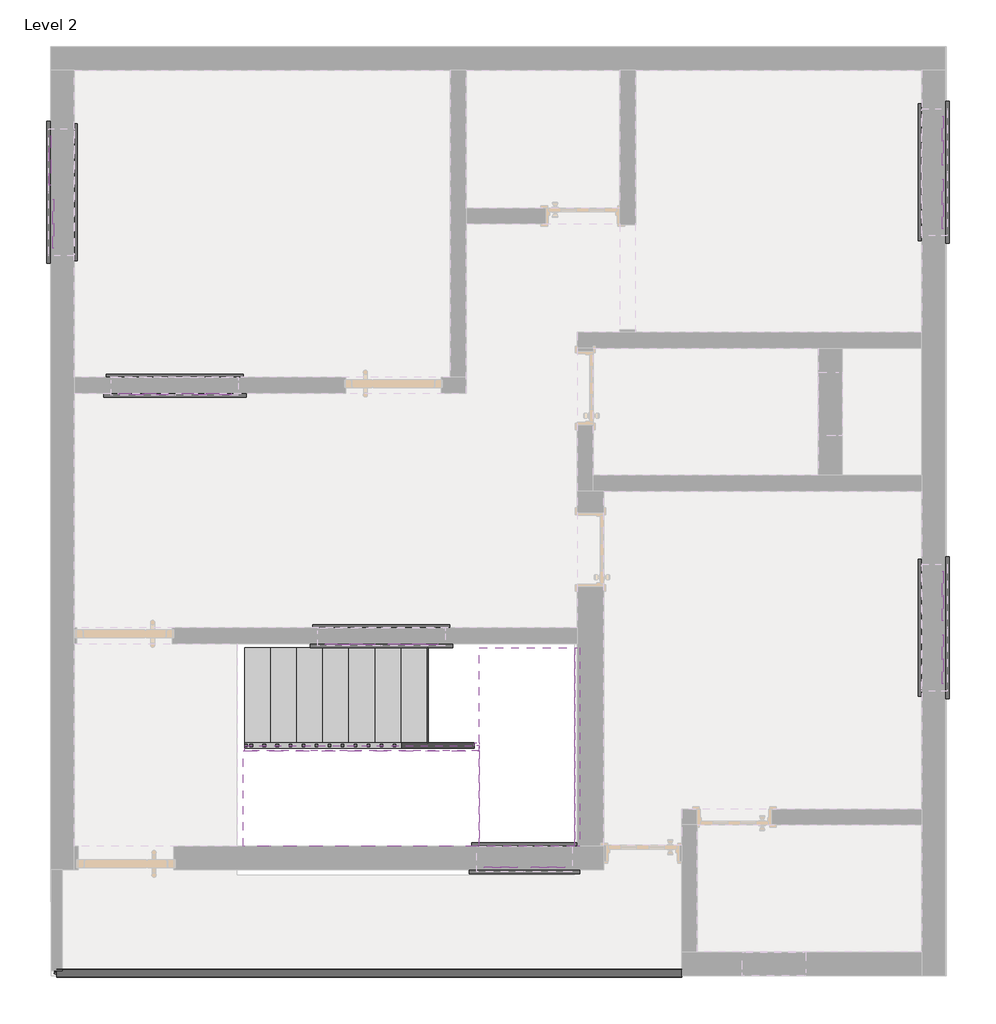
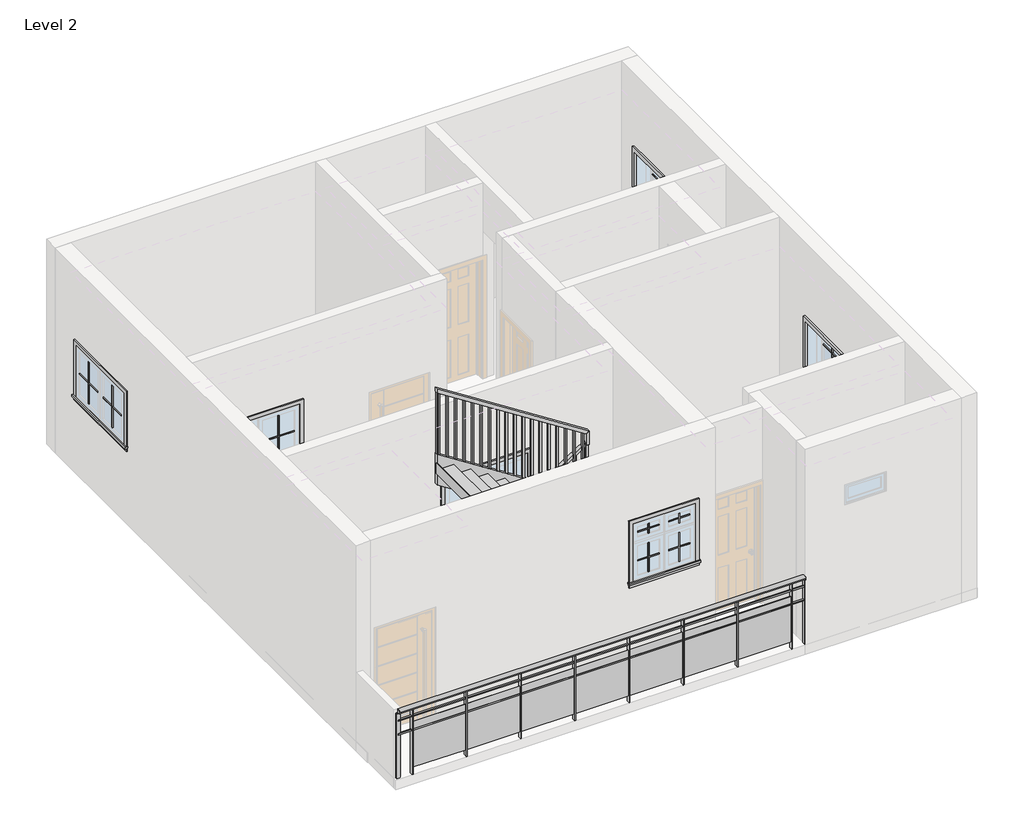
# One storey, part 2 of 2: 26 proxies, 4 members, 2 railings, 2 stair flights, 1 slab.
"""IFC4 building model written with IfcOpenShell, lengths in millimetres."""

from ifc_helpers import new_model, si_unit, point, frame, origin, place, context, project, spatial, polyline, ellipse_curve, trimmed, outline, extrude, faceted_brep, transform, mapped, element, save
from ifc_brep_helpers import plane_surface, extruded_surface, advanced_brep
from components import m_muntin_pattern_2x2_m_muntin_pattern_2x2_8d9e5da3, m_muntin_pattern_2x2_m_muntin_pattern_2x2_32a0f80e, m_muntin_pattern_2x2_m_muntin_pattern_2x2_5c9fa27a, m_muntin_pattern_2x2_m_muntin_pattern_2x2_8c7fd3cb, m_muntin_pattern_2x2_m_muntin_pattern_2x2_332c70e0, m_trim_window_exterior_flat_with_sill_3a557199, m_trim_window_exterior_flat_with_sill_8fa486dc, m_trim_window_interior_flat_picture_frame_580345df, m_trim_window_interior_flat_picture_frame_b6dd03a6, non_monolithic_landing_e1259e21, stair_flight_50mm_tread_13mm_riser_06224c7e, stair_flight_50mm_tread_13mm_riser_05b05da2

model = new_model("IFC4")

# Units and contexts
model_context = context("Model", 3, world=origin())
ifc_project = project(units=[si_unit("LENGTHUNIT", "METRE", prefix="MILLI")], contexts=[model_context])

# Site, building, storey
site = spatial("IfcSite", under=ifc_project)
building = spatial("IfcBuilding", under=site)
storey = spatial("IfcBuildingStorey", under=building, Name="Level 2", Elevation=3200.4)

# Proxies
placement = place(None, origin())
m_muntin_pattern_2x2_m_muntin_pattern_2x2_shape = m_muntin_pattern_2x2_m_muntin_pattern_2x2_8d9e5da3(model_context)
element("IfcBuildingElementProxy", 1, Name="M_Muntin Pattern_2x2 : M_Muntin Pattern_2x2", ObjectType="M_Muntin Pattern_2x2 : M_Muntin Pattern_2x2", at=placement, inside=storey, context=model_context, shape_type="MappedRepresentation", body=[
    mapped(m_muntin_pattern_2x2_m_muntin_pattern_2x2_shape, transform((-3082.7532945, -1629.5296603, 4489.45), x_axis=(0.0, -1.0, 0.0), y_axis=(1.0, 0.0, 0.0), z_axis=(0.0, 0.0, 1.0))),
])
element("IfcBuildingElementProxy", 2, Name="M_Muntin Pattern_2x2 : M_Muntin Pattern_2x2", ObjectType="M_Muntin Pattern_2x2 : M_Muntin Pattern_2x2", at=placement, inside=storey, context=model_context, shape_type="MappedRepresentation", body=[
    mapped(m_muntin_pattern_2x2_m_muntin_pattern_2x2_shape, transform((-3082.7532945, 2739.2703397, 4489.45), x_axis=(0.0, -1.0, 0.0), y_axis=(1.0, 0.0, 0.0), z_axis=(0.0, 0.0, 1.0))),
])
element("IfcBuildingElementProxy", 3, Name="M_Muntin Pattern_2x2 : M_Muntin Pattern_2x2", ObjectType="M_Muntin Pattern_2x2 : M_Muntin Pattern_2x2", at=placement, inside=storey, context=model_context, shape_type="MappedRepresentation", body=[
    mapped(m_muntin_pattern_2x2_m_muntin_pattern_2x2_shape, transform((-10161.4157945, 324.6828397, 4489.45), x_axis=(-1.0, 0.0, 0.0), y_axis=(0.0, -1.0, 0.0), z_axis=(0.0, 0.0, 1.0))),
])
element("IfcBuildingElementProxy", 4, Name="M_Muntin Pattern_2x2 : M_Muntin Pattern_2x2", ObjectType="M_Muntin Pattern_2x2 : M_Muntin Pattern_2x2", at=placement, inside=storey, context=model_context, shape_type="MappedRepresentation", body=[
    mapped(m_muntin_pattern_2x2_m_muntin_pattern_2x2_shape, transform((-11648.9032945, 1942.3453397, 4489.45), x_axis=(0.0, 1.0, 0.0), y_axis=(-1.0, 0.0, 0.0), z_axis=(0.0, 0.0, 1.0))),
])
element("IfcBuildingElementProxy", 5, Name="M_Muntin Pattern_2x2 : M_Muntin Pattern_2x2", ObjectType="M_Muntin Pattern_2x2 : M_Muntin Pattern_2x2", at=placement, inside=storey, context=model_context, shape_type="MappedRepresentation", body=[
    mapped(m_muntin_pattern_2x2_m_muntin_pattern_2x2_shape, transform((-8180.2157945, -2075.6171603, 4489.45), x_axis=(-1.0, 0.0, 0.0), y_axis=(0.0, -1.0, 0.0), z_axis=(0.0, 0.0, 1.0))),
])
m_muntin_pattern_2x2_m_muntin_pattern_2x2_2_shape = m_muntin_pattern_2x2_m_muntin_pattern_2x2_32a0f80e(model_context)
element("IfcBuildingElementProxy", 6, Name="M_Muntin Pattern_2x2 : M_Muntin Pattern_2x2", ObjectType="M_Muntin Pattern_2x2 : M_Muntin Pattern_2x2", at=placement, inside=storey, context=model_context, shape_type="MappedRepresentation", body=[
    mapped(m_muntin_pattern_2x2_m_muntin_pattern_2x2_2_shape, transform((-3082.7532945, -2235.9546603, 4489.45), x_axis=(0.0, 1.0, 0.0), y_axis=(-1.0, 0.0, 0.0), z_axis=(0.0, 0.0, 1.0))),
])
element("IfcBuildingElementProxy", 7, Name="M_Muntin Pattern_2x2 : M_Muntin Pattern_2x2", ObjectType="M_Muntin Pattern_2x2 : M_Muntin Pattern_2x2", at=placement, inside=storey, context=model_context, shape_type="MappedRepresentation", body=[
    mapped(m_muntin_pattern_2x2_m_muntin_pattern_2x2_2_shape, transform((-3082.7532945, 2132.8453397, 4489.45), x_axis=(0.0, 1.0, 0.0), y_axis=(-1.0, 0.0, 0.0), z_axis=(0.0, 0.0, 1.0))),
])
element("IfcBuildingElementProxy", 8, Name="M_Muntin Pattern_2x2 : M_Muntin Pattern_2x2", ObjectType="M_Muntin Pattern_2x2 : M_Muntin Pattern_2x2", at=placement, inside=storey, context=model_context, shape_type="MappedRepresentation", body=[
    mapped(m_muntin_pattern_2x2_m_muntin_pattern_2x2_2_shape, transform((-10767.8407945, 324.6828397, 4489.45), x_axis=(1.0, 0.0, 0.0), y_axis=(0.0, 1.0, 0.0), z_axis=(0.0, 0.0, 1.0))),
])
element("IfcBuildingElementProxy", 9, Name="M_Muntin Pattern_2x2 : M_Muntin Pattern_2x2", ObjectType="M_Muntin Pattern_2x2 : M_Muntin Pattern_2x2", at=placement, inside=storey, context=model_context, shape_type="MappedRepresentation", body=[
    mapped(m_muntin_pattern_2x2_m_muntin_pattern_2x2_2_shape, transform((-11648.9032945, 2548.7703397, 4489.45), x_axis=(0.0, -1.0, 0.0), y_axis=(1.0, 0.0, 0.0), z_axis=(0.0, 0.0, 1.0))),
])
element("IfcBuildingElementProxy", 10, Name="M_Muntin Pattern_2x2 : M_Muntin Pattern_2x2", ObjectType="M_Muntin Pattern_2x2 : M_Muntin Pattern_2x2", at=placement, inside=storey, context=model_context, shape_type="MappedRepresentation", body=[
    mapped(m_muntin_pattern_2x2_m_muntin_pattern_2x2_2_shape, transform((-8786.6407945, -2075.6171603, 4489.45), x_axis=(1.0, 0.0, 0.0), y_axis=(0.0, 1.0, 0.0), z_axis=(0.0, 0.0, 1.0))),
])
m_muntin_pattern_2x2_m_muntin_pattern_2x2_3_shape = m_muntin_pattern_2x2_m_muntin_pattern_2x2_5c9fa27a(model_context)
element("IfcBuildingElementProxy", 11, Name="M_Muntin Pattern_2x2 : M_Muntin Pattern_2x2", ObjectType="M_Muntin Pattern_2x2 : M_Muntin Pattern_2x2", at=placement, inside=storey, context=model_context, shape_type="MappedRepresentation", body=[
    mapped(m_muntin_pattern_2x2_m_muntin_pattern_2x2_3_shape, transform((-6884.8157945, -4247.3171603, 4489.45), x_axis=(-1.0, 0.0, 0.0), y_axis=(0.0, -1.0, 0.0), z_axis=(0.0, 0.0, 1.0))),
])
m_muntin_pattern_2x2_m_muntin_pattern_2x2_4_shape = m_muntin_pattern_2x2_m_muntin_pattern_2x2_8c7fd3cb(model_context)
element("IfcBuildingElementProxy", 12, Name="M_Muntin Pattern_2x2 : M_Muntin Pattern_2x2", ObjectType="M_Muntin Pattern_2x2 : M_Muntin Pattern_2x2", at=placement, inside=storey, context=model_context, shape_type="MappedRepresentation", body=[
    mapped(m_muntin_pattern_2x2_m_muntin_pattern_2x2_4_shape, transform((-7338.8407945, -4247.3171603, 4489.45), x_axis=(1.0, 0.0, 0.0), y_axis=(0.0, 1.0, 0.0), z_axis=(0.0, 0.0, 1.0))),
])
m_muntin_pattern_2x2_m_muntin_pattern_2x2_5_shape = m_muntin_pattern_2x2_m_muntin_pattern_2x2_332c70e0(model_context)
element("IfcBuildingElementProxy", 13, Name="M_Muntin Pattern_2x2 : M_Muntin Pattern_2x2", ObjectType="M_Muntin Pattern_2x2 : M_Muntin Pattern_2x2", at=placement, inside=storey, context=model_context, shape_type="MappedRepresentation", body=[
    mapped(m_muntin_pattern_2x2_m_muntin_pattern_2x2_5_shape, transform((-7338.8407945, -4247.3171603, 5089.45), x_axis=(1.0, 0.0, 0.0), y_axis=(0.0, 1.0, 0.0), z_axis=(0.0, 0.0, 1.0))),
])
element("IfcBuildingElementProxy", 14, Name="M_Muntin Pattern_2x2 : M_Muntin Pattern_2x2", ObjectType="M_Muntin Pattern_2x2 : M_Muntin Pattern_2x2", at=placement, inside=storey, context=model_context, shape_type="MappedRepresentation", body=[
    mapped(m_muntin_pattern_2x2_m_muntin_pattern_2x2_5_shape, transform((-6884.8157945, -4247.3171603, 5089.45), x_axis=(1.0, 0.0, 0.0), y_axis=(0.0, 1.0, 0.0), z_axis=(0.0, 0.0, 1.0))),
])
m_trim_window_exterior_flat_with_sill_shape = m_trim_window_exterior_flat_with_sill_3a557199(model_context)
element("IfcBuildingElementProxy", 15, Name="M_Trim-Window-Exterior-Flat : with Sill", ObjectType="M_Trim-Window-Exterior-Flat : with Sill", at=placement, inside=storey, context=model_context, shape_type="MappedRepresentation", body=[
    mapped(m_trim_window_exterior_flat_with_sill_shape, transform((-3073.2282945, -1932.7421603, 5219.6), x_axis=(0.0, 1.0, 0.0), y_axis=(0.0, 0.0, 1.0), z_axis=(1.0, 0.0, 0.0))),
])
element("IfcBuildingElementProxy", 16, Name="M_Trim-Window-Exterior-Flat : with Sill", ObjectType="M_Trim-Window-Exterior-Flat : with Sill", at=placement, inside=storey, context=model_context, shape_type="MappedRepresentation", body=[
    mapped(m_trim_window_exterior_flat_with_sill_shape, transform((-3073.2282945, 2436.0578397, 5219.6), x_axis=(0.0, 1.0, 0.0), y_axis=(0.0, 0.0, 1.0), z_axis=(1.0, 0.0, 0.0))),
])
element("IfcBuildingElementProxy", 17, Name="M_Trim-Window-Exterior-Flat : with Sill", ObjectType="M_Trim-Window-Exterior-Flat : with Sill", at=placement, inside=storey, context=model_context, shape_type="MappedRepresentation", body=[
    mapped(m_trim_window_exterior_flat_with_sill_shape, transform((-10464.6282945, 315.1578397, 5219.6), x_axis=(1.0, 0.0, 0.0), y_axis=(0.0, 0.0, 1.0), z_axis=(0.0, -1.0, 0.0))),
])
element("IfcBuildingElementProxy", 18, Name="M_Trim-Window-Exterior-Flat : with Sill", ObjectType="M_Trim-Window-Exterior-Flat : with Sill", at=placement, inside=storey, context=model_context, shape_type="MappedRepresentation", body=[
    mapped(m_trim_window_exterior_flat_with_sill_shape, transform((-11658.4282945, 2245.5578397, 5219.6), x_axis=(0.0, -1.0, 0.0), y_axis=(0.0, 0.0, 1.0), z_axis=(-1.0, 0.0, 0.0))),
])
element("IfcBuildingElementProxy", 19, Name="M_Trim-Window-Exterior-Flat : with Sill", ObjectType="M_Trim-Window-Exterior-Flat : with Sill", at=placement, inside=storey, context=model_context, shape_type="MappedRepresentation", body=[
    mapped(m_trim_window_exterior_flat_with_sill_shape, transform((-8483.4282945, -2085.1421603, 5219.6), x_axis=(1.0, 0.0, 0.0), y_axis=(0.0, 0.0, 1.0), z_axis=(0.0, -1.0, 0.0))),
])
m_trim_window_exterior_flat_with_sill_2_shape = m_trim_window_exterior_flat_with_sill_8fa486dc(model_context)
element("IfcBuildingElementProxy", 20, Name="M_Trim-Window-Exterior-Flat : with Sill", ObjectType="M_Trim-Window-Exterior-Flat : with Sill", at=placement, inside=storey, context=model_context, shape_type="MappedRepresentation", body=[
    mapped(m_trim_window_exterior_flat_with_sill_2_shape, transform((-7111.8282945, -4256.8421603, 5319.6), x_axis=(1.0, 0.0, 0.0), y_axis=(0.0, 0.0, 1.0), z_axis=(0.0, -1.0, 0.0))),
])
m_trim_window_interior_flat_picture_frame_shape = m_trim_window_interior_flat_picture_frame_580345df(model_context)
element("IfcBuildingElementProxy", 21, Name="M_Trim-Window-Interior-Flat : Picture Frame", ObjectType="M_Trim-Window-Interior-Flat : Picture Frame", at=placement, inside=storey, context=model_context, shape_type="MappedRepresentation", body=[
    mapped(m_trim_window_interior_flat_picture_frame_shape, transform((-3301.8282945, -1932.7421603, 5219.6), x_axis=(0.0, -1.0, 0.0), y_axis=(0.0, 0.0, 1.0), z_axis=(-1.0, 0.0, 0.0))),
])
element("IfcBuildingElementProxy", 22, Name="M_Trim-Window-Interior-Flat : Picture Frame", ObjectType="M_Trim-Window-Interior-Flat : Picture Frame", at=placement, inside=storey, context=model_context, shape_type="MappedRepresentation", body=[
    mapped(m_trim_window_interior_flat_picture_frame_shape, transform((-3301.8282945, 2436.0578397, 5219.6), x_axis=(0.0, -1.0, 0.0), y_axis=(0.0, 0.0, 1.0), z_axis=(-1.0, 0.0, 0.0))),
])
element("IfcBuildingElementProxy", 23, Name="M_Trim-Window-Interior-Flat : Picture Frame", ObjectType="M_Trim-Window-Interior-Flat : Picture Frame", at=placement, inside=storey, context=model_context, shape_type="MappedRepresentation", body=[
    mapped(m_trim_window_interior_flat_picture_frame_shape, transform((-10464.6282945, 467.5578397, 5219.6), x_axis=(-1.0, 0.0, 0.0), y_axis=(0.0, 0.0, 1.0), z_axis=(0.0, 1.0, 0.0))),
])
element("IfcBuildingElementProxy", 24, Name="M_Trim-Window-Interior-Flat : Picture Frame", ObjectType="M_Trim-Window-Interior-Flat : Picture Frame", at=placement, inside=storey, context=model_context, shape_type="MappedRepresentation", body=[
    mapped(m_trim_window_interior_flat_picture_frame_shape, transform((-11429.8282945, 2245.5578397, 5219.6), x_axis=(0.0, 1.0, 0.0), y_axis=(0.0, 0.0, 1.0), z_axis=(1.0, 0.0, 0.0))),
])
element("IfcBuildingElementProxy", 25, Name="M_Trim-Window-Interior-Flat : Picture Frame", ObjectType="M_Trim-Window-Interior-Flat : Picture Frame", at=placement, inside=storey, context=model_context, shape_type="MappedRepresentation", body=[
    mapped(m_trim_window_interior_flat_picture_frame_shape, transform((-8483.4282945, -1932.7421603, 5219.6), x_axis=(-1.0, 0.0, 0.0), y_axis=(0.0, 0.0, 1.0), z_axis=(0.0, 1.0, 0.0))),
])
m_trim_window_interior_flat_picture_frame_2_shape = m_trim_window_interior_flat_picture_frame_b6dd03a6(model_context)
element("IfcBuildingElementProxy", 26, Name="M_Trim-Window-Interior-Flat : Picture Frame", ObjectType="M_Trim-Window-Interior-Flat : Picture Frame", at=placement, inside=storey, context=model_context, shape_type="MappedRepresentation", body=[
    mapped(m_trim_window_interior_flat_picture_frame_2_shape, transform((-7111.8282945, -4028.2421603, 5319.6), x_axis=(-1.0, 0.0, 0.0), y_axis=(0.0, 0.0, 1.0), z_axis=(0.0, 1.0, 0.0))),
])

# Members
element("IfcMember", 27, ObjectType="Stringer - 50mm Width", at=placement, inside=storey, context=model_context, shape_type="SweptSolid", body=[
    extrude(outline(polyline([(3439.2262231, -9795.4329612), (3200.4, -9795.4329612), (3200.4, -9426.576984), (4372.4786661, -7595.4329612), (4847.4022231, -7595.4329612), (3439.2262231, -9795.4329612)])), frame((0.0, -3087.6421603, 0.0), z_axis=(0.0, 1.0, 0.0), x_axis=(0.0, 0.0, 1.0)), (0.0, 0.0, 1.0), 50.0),
])
element("IfcMember", 28, ObjectType="Stringer - 50mm Width", at=placement, inside=storey, context=model_context, shape_type="SweptSolid", body=[
    extrude(outline(polyline([(4564.5026661, -7545.4329612), (5039.4262231, -7545.4329612), (6479.6062231, -9795.4329612), (6004.6826661, -9795.4329612), (4564.5026661, -7545.4329612)])), frame((0.0, -3113.8421603, 0.0), z_axis=(0.0, 1.0, 0.0), x_axis=(0.0, 0.0, 1.0)), (0.0, 0.0, 1.0), 50.0),
])
element("IfcMember", 29, ObjectType="Stringer - 50mm Width", at=placement, inside=storey, context=model_context, shape_type="SweptSolid", body=[
    extrude(outline(polyline([(-6581.0329612, -4028.2421603), (-6631.0329612, -4028.2421603), (-6631.0329612, -2123.2421603), (-6581.0329612, -2123.2421603), (-6581.0329612, -4028.2421603)])), frame((0.0, 0.0, 4450.6), z_axis=(0.0, 0.0, 1.0), x_axis=(1.0, 0.0, 0.0)), (0.0, 0.0, 1.0), 400.0),
])
element("IfcMember", 30, ObjectType="Stringer - 50mm Width", at=placement, inside=storey, context=model_context, shape_type="SweptSolid", body=[
    extrude(outline(polyline([(-7595.4329612, -3037.6421603), (-7545.4329612, -3037.6421603), (-7545.4329612, -3063.8421603), (-7595.4329612, -3063.8421603), (-7595.4329612, -3037.6421603)])), frame((0.0, 0.0, 4450.6), z_axis=(0.0, 0.0, 1.0), x_axis=(1.0, 0.0, 0.0)), (0.0, 0.0, 1.0), 400.0),
])

# Railings
element("IfcRailing", 31, ObjectType="1100mm", at=placement, inside=storey, context=model_context, shape_type="SolidModel", body=[
    faceted_brep([(-9795.4329612, -3037.6421603, 4460.42), (-9795.4329612, -3037.6421603, 4401.0545554), (-9795.4329612, -3087.6421603, 4401.0545554), (-9795.4329612, -3087.6421603, 4460.42), (-7595.4329612, -3037.6421603, 5868.596), (-7595.4329612, -3087.6421603, 5868.596), (-7595.4329612, -3087.6421603, 5809.2305554), (-7595.4329612, -3037.6421603, 5809.2305554)], [[[0, 1, 2, 3]], [[4, 5, 6, 7]], [[1, 0, 4, 7]], [[2, 1, 7, 6]], [[3, 2, 6, 5]], [[0, 3, 5, 4]]]),
    faceted_brep([(-7545.4329612, -3037.6421603, 5900.6), (-7545.4329612, -3037.6421603, 5850.6), (-7595.4329612, -3037.6421603, 5850.6), (-7595.4329612, -3037.6421603, 5900.6), (-7545.4329612, -3063.8421603, 5900.6), (-7595.4329612, -3063.8421603, 5900.6), (-7595.4329612, -3113.8421603, 5850.6), (-7545.4329612, -3113.8421603, 5850.6)], [[[0, 1, 2, 3]], [[4, 5, 6, 7]], [[1, 0, 4, 7]], [[2, 1, 7, 6]], [[3, 2, 6, 5]], [[0, 3, 5, 4]]]),
    faceted_brep([(-7545.4329612, -3063.8421603, 5900.6), (-7545.4329612, -3113.8421603, 5850.6), (-7595.4329612, -3113.8421603, 5850.6), (-7595.4329612, -3063.8421603, 5900.6), (-7545.4329612, -3063.8421603, 6060.62), (-7595.4329612, -3063.8421603, 6033.2585554), (-7595.4329612, -3113.8421603, 6033.2585554), (-7545.4329612, -3113.8421603, 6060.62)], [[[0, 1, 2, 3]], [[4, 5, 6, 7]], [[1, 0, 4, 7]], [[2, 1, 7, 6]], [[3, 2, 6, 5]], [[0, 3, 5, 4]]]),
    faceted_brep([(-7545.4329612, -3113.8421603, 6060.62), (-7595.4329612, -3113.8421603, 6033.2585554), (-7595.4329612, -3063.8421603, 6033.2585554), (-7545.4329612, -3063.8421603, 6060.62), (-9795.4329612, -3113.8421603, 7500.8), (-9795.4329612, -3063.8421603, 7500.8), (-9795.4329612, -3063.8421603, 7441.4345554), (-9795.4329612, -3113.8421603, 7441.4345554)], [[[0, 1, 2, 3]], [[4, 5, 6, 7]], [[1, 0, 4, 7]], [[2, 1, 7, 6]], [[3, 2, 6, 5]], [[0, 3, 5, 4]]]),
    extrude(outline(polyline([(6447.6022231, -9745.4329612), (7409.4305554, -9745.4329612), (7425.4325554, -9770.4329612), (6463.6042231, -9770.4329612), (6447.6022231, -9745.4329612)])), frame((0.0, -3101.3421603, 0.0), z_axis=(0.0, 1.0, 0.0), x_axis=(0.0, 0.0, 1.0)), (0.0, 0.0, 1.0), 25.0),
    extrude(outline(polyline([(6367.5922231, -9620.4329612), (7329.4205554, -9620.4329612), (7345.4225554, -9645.4329612), (6383.5942231, -9645.4329612), (6367.5922231, -9620.4329612)])), frame((0.0, -3101.3421603, 0.0), z_axis=(0.0, 1.0, 0.0), x_axis=(0.0, 0.0, 1.0)), (0.0, 0.0, 1.0), 25.0),
    extrude(outline(polyline([(6287.5822231, -9495.4329612), (7249.4105554, -9495.4329612), (7265.4125554, -9520.4329612), (6303.5842231, -9520.4329612), (6287.5822231, -9495.4329612)])), frame((0.0, -3101.3421603, 0.0), z_axis=(0.0, 1.0, 0.0), x_axis=(0.0, 0.0, 1.0)), (0.0, 0.0, 1.0), 25.0),
    extrude(outline(polyline([(6207.5722231, -9370.4329612), (7169.4005554, -9370.4329612), (7185.4025554, -9395.4329612), (6223.5742231, -9395.4329612), (6207.5722231, -9370.4329612)])), frame((0.0, -3101.3421603, 0.0), z_axis=(0.0, 1.0, 0.0), x_axis=(0.0, 0.0, 1.0)), (0.0, 0.0, 1.0), 25.0),
    extrude(outline(polyline([(6127.5622231, -9245.4329612), (7089.3905554, -9245.4329612), (7105.3925554, -9270.4329612), (6143.5642231, -9270.4329612), (6127.5622231, -9245.4329612)])), frame((0.0, -3101.3421603, 0.0), z_axis=(0.0, 1.0, 0.0), x_axis=(0.0, 0.0, 1.0)), (0.0, 0.0, 1.0), 25.0),
    extrude(outline(polyline([(6047.5522231, -9120.4329612), (7009.3805554, -9120.4329612), (7025.3825554, -9145.4329612), (6063.5542231, -9145.4329612), (6047.5522231, -9120.4329612)])), frame((0.0, -3101.3421603, 0.0), z_axis=(0.0, 1.0, 0.0), x_axis=(0.0, 0.0, 1.0)), (0.0, 0.0, 1.0), 25.0),
    extrude(outline(polyline([(5967.5422231, -8995.4329612), (6929.3705554, -8995.4329612), (6945.3725554, -9020.4329612), (5983.5442231, -9020.4329612), (5967.5422231, -8995.4329612)])), frame((0.0, -3101.3421603, 0.0), z_axis=(0.0, 1.0, 0.0), x_axis=(0.0, 0.0, 1.0)), (0.0, 0.0, 1.0), 25.0),
    extrude(outline(polyline([(5887.5322231, -8870.4329612), (6849.3605554, -8870.4329612), (6865.3625554, -8895.4329612), (5903.5342231, -8895.4329612), (5887.5322231, -8870.4329612)])), frame((0.0, -3101.3421603, 0.0), z_axis=(0.0, 1.0, 0.0), x_axis=(0.0, 0.0, 1.0)), (0.0, 0.0, 1.0), 25.0),
    extrude(outline(polyline([(5807.5222231, -8745.4329612), (6769.3505554, -8745.4329612), (6785.3525554, -8770.4329612), (5823.5242231, -8770.4329612), (5807.5222231, -8745.4329612)])), frame((0.0, -3101.3421603, 0.0), z_axis=(0.0, 1.0, 0.0), x_axis=(0.0, 0.0, 1.0)), (0.0, 0.0, 1.0), 25.0),
    extrude(outline(polyline([(5727.5122231, -8620.4329612), (6689.3405554, -8620.4329612), (6705.3425554, -8645.4329612), (5743.5142231, -8645.4329612), (5727.5122231, -8620.4329612)])), frame((0.0, -3101.3421603, 0.0), z_axis=(0.0, 1.0, 0.0), x_axis=(0.0, 0.0, 1.0)), (0.0, 0.0, 1.0), 25.0),
    extrude(outline(polyline([(5647.5022231, -8495.4329612), (6609.3305554, -8495.4329612), (6625.3325554, -8520.4329612), (5663.5042231, -8520.4329612), (5647.5022231, -8495.4329612)])), frame((0.0, -3101.3421603, 0.0), z_axis=(0.0, 1.0, 0.0), x_axis=(0.0, 0.0, 1.0)), (0.0, 0.0, 1.0), 25.0),
    extrude(outline(polyline([(5567.4922231, -8370.4329612), (6529.3205554, -8370.4329612), (6545.3225554, -8395.4329612), (5583.4942231, -8395.4329612), (5567.4922231, -8370.4329612)])), frame((0.0, -3101.3421603, 0.0), z_axis=(0.0, 1.0, 0.0), x_axis=(0.0, 0.0, 1.0)), (0.0, 0.0, 1.0), 25.0),
    extrude(outline(polyline([(5487.4822231, -8245.4329612), (6449.3105554, -8245.4329612), (6465.3125554, -8270.4329612), (5503.4842231, -8270.4329612), (5487.4822231, -8245.4329612)])), frame((0.0, -3101.3421603, 0.0), z_axis=(0.0, 1.0, 0.0), x_axis=(0.0, 0.0, 1.0)), (0.0, 0.0, 1.0), 25.0),
    extrude(outline(polyline([(5407.4722231, -8120.4329612), (6369.3005554, -8120.4329612), (6385.3025554, -8145.4329612), (5423.4742231, -8145.4329612), (5407.4722231, -8120.4329612)])), frame((0.0, -3101.3421603, 0.0), z_axis=(0.0, 1.0, 0.0), x_axis=(0.0, 0.0, 1.0)), (0.0, 0.0, 1.0), 25.0),
    extrude(outline(polyline([(5327.4622231, -7995.4329612), (6289.2905554, -7995.4329612), (6305.2925554, -8020.4329612), (5343.4642231, -8020.4329612), (5327.4622231, -7995.4329612)])), frame((0.0, -3101.3421603, 0.0), z_axis=(0.0, 1.0, 0.0), x_axis=(0.0, 0.0, 1.0)), (0.0, 0.0, 1.0), 25.0),
    extrude(outline(polyline([(5247.4522231, -7870.4329612), (6209.2805554, -7870.4329612), (6225.2825554, -7895.4329612), (5263.4542231, -7895.4329612), (5247.4522231, -7870.4329612)])), frame((0.0, -3101.3421603, 0.0), z_axis=(0.0, 1.0, 0.0), x_axis=(0.0, 0.0, 1.0)), (0.0, 0.0, 1.0), 25.0),
    extrude(outline(polyline([(5167.4422231, -7745.4329612), (6129.2705554, -7745.4329612), (6145.2725554, -7770.4329612), (5183.4442231, -7770.4329612), (5167.4422231, -7745.4329612)])), frame((0.0, -3101.3421603, 0.0), z_axis=(0.0, 1.0, 0.0), x_axis=(0.0, 0.0, 1.0)), (0.0, 0.0, 1.0), 25.0),
    extrude(outline(polyline([(5087.4322231, -7620.4329612), (6049.2605554, -7620.4329612), (6065.2625554, -7645.4329612), (5103.4342231, -7645.4329612), (5087.4322231, -7620.4329612)])), frame((0.0, -3101.3421603, 0.0), z_axis=(0.0, 1.0, 0.0), x_axis=(0.0, 0.0, 1.0)), (0.0, 0.0, 1.0), 25.0),
    extrude(outline(polyline([(5793.2285554, -7620.4329612), (4831.4002231, -7620.4329612), (4847.4022231, -7595.4329612), (5809.2305554, -7595.4329612), (5793.2285554, -7620.4329612)])), frame((0.0, -3075.1421603, 0.0), z_axis=(0.0, 1.0, 0.0), x_axis=(0.0, 0.0, 1.0)), (0.0, 0.0, 1.0), 25.0),
    extrude(outline(polyline([(5713.2185554, -7745.4329612), (4751.3902231, -7745.4329612), (4767.3922231, -7720.4329612), (5729.2205554, -7720.4329612), (5713.2185554, -7745.4329612)])), frame((0.0, -3075.1421603, 0.0), z_axis=(0.0, 1.0, 0.0), x_axis=(0.0, 0.0, 1.0)), (0.0, 0.0, 1.0), 25.0),
    extrude(outline(polyline([(5633.2085554, -7870.4329612), (4671.3802231, -7870.4329612), (4687.3822231, -7845.4329612), (5649.2105554, -7845.4329612), (5633.2085554, -7870.4329612)])), frame((0.0, -3075.1421603, 0.0), z_axis=(0.0, 1.0, 0.0), x_axis=(0.0, 0.0, 1.0)), (0.0, 0.0, 1.0), 25.0),
    extrude(outline(polyline([(5553.1985554, -7995.4329612), (4591.3702231, -7995.4329612), (4607.3722231, -7970.4329612), (5569.2005554, -7970.4329612), (5553.1985554, -7995.4329612)])), frame((0.0, -3075.1421603, 0.0), z_axis=(0.0, 1.0, 0.0), x_axis=(0.0, 0.0, 1.0)), (0.0, 0.0, 1.0), 25.0),
    extrude(outline(polyline([(5473.1885554, -8120.4329612), (4511.3602231, -8120.4329612), (4527.3622231, -8095.4329612), (5489.1905554, -8095.4329612), (5473.1885554, -8120.4329612)])), frame((0.0, -3075.1421603, 0.0), z_axis=(0.0, 1.0, 0.0), x_axis=(0.0, 0.0, 1.0)), (0.0, 0.0, 1.0), 25.0),
    extrude(outline(polyline([(5393.1785554, -8245.4329612), (4431.3502231, -8245.4329612), (4447.3522231, -8220.4329612), (5409.1805554, -8220.4329612), (5393.1785554, -8245.4329612)])), frame((0.0, -3075.1421603, 0.0), z_axis=(0.0, 1.0, 0.0), x_axis=(0.0, 0.0, 1.0)), (0.0, 0.0, 1.0), 25.0),
    extrude(outline(polyline([(5313.1685554, -8370.4329612), (4351.3402231, -8370.4329612), (4367.3422231, -8345.4329612), (5329.1705554, -8345.4329612), (5313.1685554, -8370.4329612)])), frame((0.0, -3075.1421603, 0.0), z_axis=(0.0, 1.0, 0.0), x_axis=(0.0, 0.0, 1.0)), (0.0, 0.0, 1.0), 25.0),
    extrude(outline(polyline([(5233.1585554, -8495.4329612), (4271.3302231, -8495.4329612), (4287.3322231, -8470.4329612), (5249.1605554, -8470.4329612), (5233.1585554, -8495.4329612)])), frame((0.0, -3075.1421603, 0.0), z_axis=(0.0, 1.0, 0.0), x_axis=(0.0, 0.0, 1.0)), (0.0, 0.0, 1.0), 25.0),
    extrude(outline(polyline([(5153.1485554, -8620.4329612), (4191.3202231, -8620.4329612), (4207.3222231, -8595.4329612), (5169.1505554, -8595.4329612), (5153.1485554, -8620.4329612)])), frame((0.0, -3075.1421603, 0.0), z_axis=(0.0, 1.0, 0.0), x_axis=(0.0, 0.0, 1.0)), (0.0, 0.0, 1.0), 25.0),
    extrude(outline(polyline([(5073.1385554, -8745.4329612), (4111.3102231, -8745.4329612), (4127.3122231, -8720.4329612), (5089.1405554, -8720.4329612), (5073.1385554, -8745.4329612)])), frame((0.0, -3075.1421603, 0.0), z_axis=(0.0, 1.0, 0.0), x_axis=(0.0, 0.0, 1.0)), (0.0, 0.0, 1.0), 25.0),
    extrude(outline(polyline([(4993.1285554, -8870.4329612), (4031.3002231, -8870.4329612), (4047.3022231, -8845.4329612), (5009.1305554, -8845.4329612), (4993.1285554, -8870.4329612)])), frame((0.0, -3075.1421603, 0.0), z_axis=(0.0, 1.0, 0.0), x_axis=(0.0, 0.0, 1.0)), (0.0, 0.0, 1.0), 25.0),
    extrude(outline(polyline([(4913.1185554, -8995.4329612), (3951.2902231, -8995.4329612), (3967.2922231, -8970.4329612), (4929.1205554, -8970.4329612), (4913.1185554, -8995.4329612)])), frame((0.0, -3075.1421603, 0.0), z_axis=(0.0, 1.0, 0.0), x_axis=(0.0, 0.0, 1.0)), (0.0, 0.0, 1.0), 25.0),
    extrude(outline(polyline([(4833.1085554, -9120.4329612), (3871.2802231, -9120.4329612), (3887.2822231, -9095.4329612), (4849.1105554, -9095.4329612), (4833.1085554, -9120.4329612)])), frame((0.0, -3075.1421603, 0.0), z_axis=(0.0, 1.0, 0.0), x_axis=(0.0, 0.0, 1.0)), (0.0, 0.0, 1.0), 25.0),
    extrude(outline(polyline([(4753.0985554, -9245.4329612), (3791.2702231, -9245.4329612), (3807.2722231, -9220.4329612), (4769.1005554, -9220.4329612), (4753.0985554, -9245.4329612)])), frame((0.0, -3075.1421603, 0.0), z_axis=(0.0, 1.0, 0.0), x_axis=(0.0, 0.0, 1.0)), (0.0, 0.0, 1.0), 25.0),
    extrude(outline(polyline([(4673.0885554, -9370.4329612), (3711.2602231, -9370.4329612), (3727.2622231, -9345.4329612), (4689.0905554, -9345.4329612), (4673.0885554, -9370.4329612)])), frame((0.0, -3075.1421603, 0.0), z_axis=(0.0, 1.0, 0.0), x_axis=(0.0, 0.0, 1.0)), (0.0, 0.0, 1.0), 25.0),
    extrude(outline(polyline([(4593.0785554, -9495.4329612), (3631.2502231, -9495.4329612), (3647.2522231, -9470.4329612), (4609.0805554, -9470.4329612), (4593.0785554, -9495.4329612)])), frame((0.0, -3075.1421603, 0.0), z_axis=(0.0, 1.0, 0.0), x_axis=(0.0, 0.0, 1.0)), (0.0, 0.0, 1.0), 25.0),
    extrude(outline(polyline([(4513.0685554, -9620.4329612), (3551.2402231, -9620.4329612), (3567.2422231, -9595.4329612), (4529.0705554, -9595.4329612), (4513.0685554, -9620.4329612)])), frame((0.0, -3075.1421603, 0.0), z_axis=(0.0, 1.0, 0.0), x_axis=(0.0, 0.0, 1.0)), (0.0, 0.0, 1.0), 25.0),
    extrude(outline(polyline([(4433.0585554, -9745.4329612), (3471.2302231, -9745.4329612), (3487.2322231, -9720.4329612), (4449.0605554, -9720.4329612), (4433.0585554, -9745.4329612)])), frame((0.0, -3075.1421603, 0.0), z_axis=(0.0, 1.0, 0.0), x_axis=(0.0, 0.0, 1.0)), (0.0, 0.0, 1.0), 25.0),
    extrude(outline(polyline([(-3076.3421603, 5850.6), (-3076.3421603, 5047.4272231), (-3101.3421603, 5063.4292231), (-3101.3421603, 5850.6), (-3076.3421603, 5850.6)])), frame((-7582.9329612, 0.0, 0.0), z_axis=(1.0, 0.0, 0.0), x_axis=(0.0, 1.0, 0.0)), (0.0, 0.0, 1.0), 25.0),
    extrude(outline(polyline([(5817.2315554, -7582.9329612), (4850.6, -7582.9329612), (4850.6, -7557.9329612), (5833.2335554, -7557.9329612), (5817.2315554, -7582.9329612)])), frame((0.0, -3075.1421603, 0.0), z_axis=(0.0, 1.0, 0.0), x_axis=(0.0, 0.0, 1.0)), (0.0, 0.0, 1.0), 25.0),
    extrude(outline(polyline([(6463.6042231, -9770.4329612), (7425.4325554, -9770.4329612), (7441.4345554, -9795.4329612), (6479.6062231, -9795.4329612), (6463.6042231, -9770.4329612)])), frame((0.0, -3101.3421603, 0.0), z_axis=(0.0, 1.0, 0.0), x_axis=(0.0, 0.0, 1.0)), (0.0, 0.0, 1.0), 25.0),
    extrude(outline(polyline([(4401.0545554, -9795.4329612), (3439.2262231, -9795.4329612), (3455.2282231, -9770.4329612), (4417.0565554, -9770.4329612), (4401.0545554, -9795.4329612)])), frame((0.0, -3075.1421603, 0.0), z_axis=(0.0, 1.0, 0.0), x_axis=(0.0, 0.0, 1.0)), (0.0, 0.0, 1.0), 25.0),
])
element("IfcRailing", 32, ObjectType="Glass Panel - Bottom Fill", at=placement, inside=storey, context=model_context, shape_type="SolidModel", body=[
    advanced_brep(
    [(-11598.8329612, -5208.0513952, 4394.2), (-11598.8329612, -5288.0513952, 4394.2), (-5604.4329612, -5208.0513952, 4394.2), (-5604.4329612, -5288.0513952, 4394.2)],
    [
        (0, 1, ellipse_curve(frame((-11598.8329612, -5248.0513952, 4394.2), z_axis=(-1.0, 0.0, 0.0), x_axis=(0.0, -1.0, 0.0)), 40.0, 30.0)),
        (1, 0, ellipse_curve(frame((-11598.8329612, -5248.0513952, 4394.2), z_axis=(-1.0, 0.0, 0.0), x_axis=(0.0, -1.0, 0.0)), 40.0, 30.0)),
        (2, 3, ellipse_curve(frame((-5604.4329612, -5248.0513952, 4394.2), z_axis=(1.0, 0.0, 0.0), x_axis=(0.0, -1.0, 0.0)), 40.0, 30.0)),
        (3, 2, ellipse_curve(frame((-5604.4329612, -5248.0513952, 4394.2), z_axis=(1.0, 0.0, 0.0), x_axis=(0.0, -1.0, 0.0)), 40.0, 30.0)),
        (0, 2),
        (3, 1),
    ],
    [
        plane_surface(frame((-11598.8329612, -5248.0513952, 4394.2), z_axis=(-1.0, 0.0, 0.0), x_axis=(0.0, 1.0, 0.0))),
        plane_surface(frame((-5604.4329612, -5248.0513952, 4394.2), z_axis=(1.0, 0.0, 0.0), x_axis=(0.0, 1.0, 0.0))),
        extruded_surface(trimmed(ellipse_curve(frame((-5604.4329612, -5248.0513952, 4394.2), z_axis=(-1.0, 0.0, 0.0), x_axis=(0.0, -1.0, 0.0)), 40.0, 30.0), [point((-5604.4329612, -5208.0513952, 4394.2))], [point((-5604.4329612, -5288.0513952, 4394.2))], True, "CARTESIAN"), (-5994.4, 0.0, 0.0), 5994.4),
        extruded_surface(trimmed(ellipse_curve(frame((-5604.4329612, -5248.0513952, 4394.2), z_axis=(-1.0, 0.0, 0.0), x_axis=(0.0, -1.0, 0.0)), 40.0, 30.0), [point((-5604.4329612, -5288.0513952, 4394.2))], [point((-5604.4329612, -5208.0513952, 4394.2))], True, "CARTESIAN"), (-5994.4, 0.0, 0.0), 5994.4),
    ],
    [
        (0, [[1, 2]]),
        (1, [[3, 4]]),
        (2, [[-1, 5, -4, 6]]),
        (3, [[-2, -6, -3, -5]]),
    ],
),
    faceted_brep([(-11608.8329612, -5222.0421603, 4267.2), (-11588.8329612, -5222.0421603, 4267.2), (-11588.8329612, -5222.0421603, 4247.2), (-11608.8329612, -5222.0421603, 4247.2), (-11608.8329612, -5257.4421603, 4267.2), (-11588.8329612, -5237.4421603, 4267.2), (-11588.8329612, -5237.4421603, 4247.2), (-11608.8329612, -5257.4421603, 4247.2), (-5604.4329612, -5257.4421603, 4267.2), (-5604.4329612, -5257.4421603, 4247.2), (-5604.4329612, -5237.4421603, 4247.2), (-5604.4329612, -5237.4421603, 4267.2)], [[[0, 1, 2, 3]], [[1, 0, 4, 5]], [[2, 1, 5, 6]], [[3, 2, 6, 7]], [[0, 3, 7, 4]], [[8, 9, 10, 11]], [[5, 4, 8, 11]], [[6, 5, 11, 10]], [[7, 6, 10, 9]], [[4, 7, 9, 8]]]),
    faceted_brep([(-11608.8329612, -5222.0421603, 4052.7882813), (-11588.8329612, -5222.0421603, 4052.7882813), (-11588.8329612, -5222.0421603, 4032.7882813), (-11608.8329612, -5222.0421603, 4032.7882813), (-11608.8329612, -5257.4421603, 4052.7882813), (-11588.8329612, -5237.4421603, 4052.7882813), (-11588.8329612, -5237.4421603, 4032.7882813), (-11608.8329612, -5257.4421603, 4032.7882813), (-5604.4329612, -5257.4421603, 4052.7882813), (-5604.4329612, -5257.4421603, 4032.7882813), (-5604.4329612, -5237.4421603, 4032.7882813), (-5604.4329612, -5237.4421603, 4052.7882813)], [[[0, 1, 2, 3]], [[1, 0, 4, 5]], [[2, 1, 5, 6]], [[3, 2, 6, 7]], [[0, 3, 7, 4]], [[8, 9, 10, 11]], [[5, 4, 8, 11]], [[6, 5, 11, 10]], [[7, 6, 10, 9]], [[4, 7, 9, 8]]]),
    extrude(outline(polyline([(-5807.6329612, -5222.4421603), (-5795.6329612, -5222.4421603), (-5795.6329612, -5272.4421603), (-5807.6329612, -5272.4421603), (-5807.6329612, -5222.4421603)])), frame((0.0, 0.0, 3352.8), z_axis=(0.0, 0.0, 1.0), x_axis=(1.0, 0.0, 0.0)), (0.0, 0.0, 1.0), 1011.4),
    extrude(outline(polyline([(-6601.6329612, -5249.1669704), (-5801.6329612, -5249.1669704), (-5801.6329612, -5254.1669704), (-6601.6329612, -5254.1669704), (-6601.6329612, -5249.1669704)])), frame((0.0, 0.0, 3452.8), z_axis=(0.0, 0.0, 1.0), x_axis=(1.0, 0.0, 0.0)), (0.0, 0.0, 1.0), 714.4),
    extrude(outline(polyline([(-6607.6329612, -5222.4421603), (-6595.6329612, -5222.4421603), (-6595.6329612, -5272.4421603), (-6607.6329612, -5272.4421603), (-6607.6329612, -5222.4421603)])), frame((0.0, 0.0, 3352.8), z_axis=(0.0, 0.0, 1.0), x_axis=(1.0, 0.0, 0.0)), (0.0, 0.0, 1.0), 1011.4),
    extrude(outline(polyline([(-7401.6329612, -5249.1669704), (-6601.6329612, -5249.1669704), (-6601.6329612, -5254.1669704), (-7401.6329612, -5254.1669704), (-7401.6329612, -5249.1669704)])), frame((0.0, 0.0, 3452.8), z_axis=(0.0, 0.0, 1.0), x_axis=(1.0, 0.0, 0.0)), (0.0, 0.0, 1.0), 714.4),
    extrude(outline(polyline([(-7407.6329612, -5222.4421603), (-7395.6329612, -5222.4421603), (-7395.6329612, -5272.4421603), (-7407.6329612, -5272.4421603), (-7407.6329612, -5222.4421603)])), frame((0.0, 0.0, 3352.8), z_axis=(0.0, 0.0, 1.0), x_axis=(1.0, 0.0, 0.0)), (0.0, 0.0, 1.0), 1011.4),
    extrude(outline(polyline([(-8201.6329612, -5249.1669704), (-7401.6329612, -5249.1669704), (-7401.6329612, -5254.1669704), (-8201.6329612, -5254.1669704), (-8201.6329612, -5249.1669704)])), frame((0.0, 0.0, 3452.8), z_axis=(0.0, 0.0, 1.0), x_axis=(1.0, 0.0, 0.0)), (0.0, 0.0, 1.0), 714.4),
    extrude(outline(polyline([(-8207.6329612, -5222.4421603), (-8195.6329612, -5222.4421603), (-8195.6329612, -5272.4421603), (-8207.6329612, -5272.4421603), (-8207.6329612, -5222.4421603)])), frame((0.0, 0.0, 3352.8), z_axis=(0.0, 0.0, 1.0), x_axis=(1.0, 0.0, 0.0)), (0.0, 0.0, 1.0), 1011.4),
    extrude(outline(polyline([(-9001.6329612, -5249.1669704), (-8201.6329612, -5249.1669704), (-8201.6329612, -5254.1669704), (-9001.6329612, -5254.1669704), (-9001.6329612, -5249.1669704)])), frame((0.0, 0.0, 3452.8), z_axis=(0.0, 0.0, 1.0), x_axis=(1.0, 0.0, 0.0)), (0.0, 0.0, 1.0), 714.4),
    extrude(outline(polyline([(-9007.6329612, -5222.4421603), (-8995.6329612, -5222.4421603), (-8995.6329612, -5272.4421603), (-9007.6329612, -5272.4421603), (-9007.6329612, -5222.4421603)])), frame((0.0, 0.0, 3352.8), z_axis=(0.0, 0.0, 1.0), x_axis=(1.0, 0.0, 0.0)), (0.0, 0.0, 1.0), 1011.4),
    extrude(outline(polyline([(-9801.6329612, -5249.1669704), (-9001.6329612, -5249.1669704), (-9001.6329612, -5254.1669704), (-9801.6329612, -5254.1669704), (-9801.6329612, -5249.1669704)])), frame((0.0, 0.0, 3452.8), z_axis=(0.0, 0.0, 1.0), x_axis=(1.0, 0.0, 0.0)), (0.0, 0.0, 1.0), 714.4),
    extrude(outline(polyline([(-9807.6329612, -5222.4421603), (-9795.6329612, -5222.4421603), (-9795.6329612, -5272.4421603), (-9807.6329612, -5272.4421603), (-9807.6329612, -5222.4421603)])), frame((0.0, 0.0, 3352.8), z_axis=(0.0, 0.0, 1.0), x_axis=(1.0, 0.0, 0.0)), (0.0, 0.0, 1.0), 1011.4),
    extrude(outline(polyline([(-10601.6329612, -5249.1669704), (-9801.6329612, -5249.1669704), (-9801.6329612, -5254.1669704), (-10601.6329612, -5254.1669704), (-10601.6329612, -5249.1669704)])), frame((0.0, 0.0, 3452.8), z_axis=(0.0, 0.0, 1.0), x_axis=(1.0, 0.0, 0.0)), (0.0, 0.0, 1.0), 714.4),
    extrude(outline(polyline([(-10607.6329612, -5222.4421603), (-10595.6329612, -5222.4421603), (-10595.6329612, -5272.4421603), (-10607.6329612, -5272.4421603), (-10607.6329612, -5222.4421603)])), frame((0.0, 0.0, 3352.8), z_axis=(0.0, 0.0, 1.0), x_axis=(1.0, 0.0, 0.0)), (0.0, 0.0, 1.0), 1011.4),
    extrude(outline(polyline([(-11401.6329612, -5249.1669704), (-10601.6329612, -5249.1669704), (-10601.6329612, -5254.1669704), (-11401.6329612, -5254.1669704), (-11401.6329612, -5249.1669704)])), frame((0.0, 0.0, 3452.8), z_axis=(0.0, 0.0, 1.0), x_axis=(1.0, 0.0, 0.0)), (0.0, 0.0, 1.0), 714.4),
    extrude(outline(polyline([(-11407.6329612, -5222.4421603), (-11395.6329612, -5222.4421603), (-11395.6329612, -5272.4421603), (-11407.6329612, -5272.4421603), (-11407.6329612, -5222.4421603)])), frame((0.0, 0.0, 3352.8), z_axis=(0.0, 0.0, 1.0), x_axis=(1.0, 0.0, 0.0)), (0.0, 0.0, 1.0), 1011.4),
    extrude(outline(polyline([(-11573.8329612, -5241.4421603), (-11573.8329612, -5253.4421603), (-11623.8329612, -5253.4421603), (-11623.8329612, -5241.4421603), (-11573.8329612, -5241.4421603)])), frame((0.0, 0.0, 3352.8), z_axis=(0.0, 0.0, 1.0), x_axis=(1.0, 0.0, 0.0)), (0.0, 0.0, 1.0), 1011.4),
    extrude(outline(polyline([(-5612.4329612, -5222.4421603), (-5600.4329612, -5222.4421603), (-5600.4329612, -5272.4421603), (-5612.4329612, -5272.4421603), (-5612.4329612, -5222.4421603)])), frame((0.0, 0.0, 3352.8), z_axis=(0.0, 0.0, 1.0), x_axis=(1.0, 0.0, 0.0)), (0.0, 0.0, 1.0), 1011.4),
    extrude(outline(polyline([(-11573.8329612, -5218.0421603), (-11573.8329612, -5230.0421603), (-11623.8329612, -5230.0421603), (-11623.8329612, -5218.0421603), (-11573.8329612, -5218.0421603)])), frame((0.0, 0.0, 3352.8), z_axis=(0.0, 0.0, 1.0), x_axis=(1.0, 0.0, 0.0)), (0.0, 0.0, 1.0), 1011.4),
])

# Slab
non_monolithic_landing_shape = non_monolithic_landing_e1259e21(model_context)
element("IfcSlab", 33, ObjectType="Non-Monolithic Landing", at=placement, inside=storey, context=model_context, shape_type="MappedRepresentation", body=[
    mapped(non_monolithic_landing_shape, transform((0.0, 0.0, 0.0), x_axis=(1.0, 0.0, 0.0), y_axis=(0.0, 1.0, 0.0), z_axis=(0.0, 0.0, 1.0))),
])

# Stair flights
stair_flight_50mm_tread_13mm_riser_shape = stair_flight_50mm_tread_13mm_riser_06224c7e(model_context)
element("IfcStairFlight", 34, ObjectType="50mm Tread 13mm Riser", at=placement, inside=storey, context=model_context, shape_type="MappedRepresentation", body=[
    mapped(stair_flight_50mm_tread_13mm_riser_shape, transform((0.0, 0.0, 0.0), x_axis=(1.0, 0.0, 0.0), y_axis=(0.0, 1.0, 0.0), z_axis=(0.0, 0.0, 1.0))),
])
stair_flight_50mm_tread_13mm_riser_2_shape = stair_flight_50mm_tread_13mm_riser_05b05da2(model_context)
element("IfcStairFlight", 35, ObjectType="50mm Tread 13mm Riser", at=placement, inside=storey, context=model_context, shape_type="MappedRepresentation", body=[
    mapped(stair_flight_50mm_tread_13mm_riser_2_shape, transform((0.0, 0.0, 0.0), x_axis=(1.0, 0.0, 0.0), y_axis=(0.0, 1.0, 0.0), z_axis=(0.0, 0.0, 1.0))),
])

save(model, "model.ifc")

# Revit data of these elements
# Type "M_Muntin Pattern_2x2 : M_Muntin Pattern_2x2"
#   Width [instance default] = 3' - 11.24409"
#   Thickness = 0' - 0 1/2"
#   Height [instance default] = 3' - 11.24409"
#   Distance = 0' - 0 3/4"
#   Interior Material [instance default] = none
#   Exterior Material [instance default] = none
#   Default Elevation = 0
# Type "M_Trim-Window-Exterior-Flat : with Sill"
#   Trim Width = 0' - 2.3622"
#   Trim Thickness_Picture Frame = 0' - 1.1811"
#   Trim Thickness_with Sill = 0' - 0 3/4"
#   Sill Thickness = 0' - 1.1811"
#   Opening Width [instance default] = 1' - 11.62205"
#   Opening Height [instance default] = 2' - 11.43307"
#   Default Elevation = 3' - 11.24409"
#   Sill = yes
#   Picture Frame = no
#   Trim Material [instance default] = none
# Type "M_Trim-Window-Interior-Flat : Picture Frame"
#   Trim Thickness_Picture Frame = 0' - 1.1811"
#   Trim Width = 0' - 2.3622"
#   Trim Thickness_with Sill = 0' - 0.7874"
#   Sill Thickness = 0' - 1.1811"
#   Opening Width [instance default] = 1' - 11.62205"
#   Opening Height [instance default] = 2' - 11.43307"
#   Default Elevation = 3' - 11.24409"
#   Sill = no
#   Picture Frame = yes
#   Trim Material [instance default] = none
# Type "1100mm"
#   built-in parameter 1008612 = 0.019685 (stored number, unit not read)
#   built-in parameter 1008611 = 0.019685 (stored number, unit not read)
#   built-in parameter 1008609 = 0.902231 (stored number, unit not read)
#   built-in parameter 1008604 = 0.19685 (stored number, unit not read)
#   built-in parameter 1008603 = 0.164042 (stored number, unit not read)
#   Railing Height = 3' - 7.30709"
#   built-in parameter 1008630 = 2
#   built-in parameter 1008610 = 2
#   built-in parameter 1008608 = 1
#   built-in parameter 1008618 = M_Baluster - Square : 25mm
# Type "Glass Panel - Bottom Fill"
#   built-in parameter 1008612 = 0.019685 (stored number, unit not read)
#   built-in parameter 1008611 = 0.019685 (stored number, unit not read)
#   built-in parameter 1008609 = 0.902231 (stored number, unit not read)
#   built-in parameter 1008604 = 0.19685 (stored number, unit not read)
#   built-in parameter 1008603 = 0.164042 (stored number, unit not read)
#   Railing Height = 3' - 5"
#   built-in parameter 1008630 = 2
#   built-in parameter 1008610 = 2
# Elements 1, 2, 3, 4, 5, 6, 7, 8, 9, 10 (IfcBuildingElementProxy, "M_Muntin Pattern_2x2 : M_Muntin Pattern_2x2")
#   Width = 1' - 6 5/8"
#   Height = 2' - 1.99606"
#   Interior Material = Wood - Stained
#   Exterior Material = Clad - White
#   Phase Created = New Construction
#   Materials on its faces: "Clad - White", "Wood - Stained"
# Elements 11, 12 (IfcBuildingElementProxy, "M_Muntin Pattern_2x2 : M_Muntin Pattern_2x2")
#   Width = 1' - 0 5/8"
#   Height = 1' - 6.12205"
#   Interior Material = Wood - Stained
#   Exterior Material = Clad - White
#   Phase Created = New Construction
#   Materials on its faces: "Clad - White", "Wood - Stained"
# Elements 13, 14 (IfcBuildingElementProxy, "M_Muntin Pattern_2x2 : M_Muntin Pattern_2x2")
#   Width = 1' - 0 5/8"
#   Height = 0' - 6.31102"
#   Interior Material = Wood - Stained
#   Exterior Material = Clad - White
#   Phase Created = New Construction
#   Materials on its faces: "Clad - White", "Wood - Stained"
# Elements 15, 16, 17, 18, 19 (IfcBuildingElementProxy, "M_Trim-Window-Exterior-Flat : with Sill")
#   Opening Width = 4' - 0"
#   Opening Height = 2' - 7.49606"
#   Trim Material = Clad - White
#   Phase Created = New Construction
#   Materials on its faces: "Clad - White"
# Element 20 (IfcBuildingElementProxy, "M_Trim-Window-Exterior-Flat : with Sill")
#   Opening Width = 3' - 0"
#   Opening Height = 2' - 11.43307"
#   Trim Material = Clad - White
#   Phase Created = New Construction
#   Materials on its faces: "Clad - White"
# Elements 21, 22, 23, 24, 25 (IfcBuildingElementProxy, "M_Trim-Window-Interior-Flat : Picture Frame")
#   Opening Width = 4' - 0"
#   Opening Height = 2' - 7.49606"
#   Trim Material = Wood - Stained
#   Phase Created = New Construction
#   Materials on its faces: "Wood - Stained"
# Element 26 (IfcBuildingElementProxy, "M_Trim-Window-Interior-Flat : Picture Frame")
#   Opening Width = 3' - 0"
#   Opening Height = 2' - 11.43307"
#   Trim Material = Wood - Stained
#   Phase Created = New Construction
#   Materials on its faces: "Wood - Stained"
# Elements 27, 28, 29, 30 (IfcMember, "Stringer - 50mm Width")
#   Phase Created = New Construction
# Element 31 (IfcRailing, "1100mm")
#   Phase Created = New Construction
# Element 32 (IfcRailing, "Glass Panel - Bottom Fill")
#   built-in parameter 1008621 = 0.5 (stored number, unit not read)
#   Phase Created = New Construction
#   Materials on its faces: "Metal - Stainless Steel,Polished", "Glass"
# Element 33 (IfcSlab, "Non-Monolithic Landing")
#   Phase Created = New Construction
# Elements 34, 35 (IfcStairFlight, "50mm Tread 13mm Riser")
#   Phase Created = New Construction
# Materials
#   "Clad - White": class "Wood", colour RGB 242 242 238, transparency 0, Cost = 0
#   "Wood - Stained": class "Wood", colour RGB 224 178 126, transparency 0, Cost = 0
#   "Metal - Stainless Steel,Polished": class "Metal", colour RGB 236 239 239, transparency 0, Cost = 0
#   "Glass": class "Glass", colour RGB 0 128 192, transparency 0.9, Description = "Soda Lime Glass", Cost = 0
